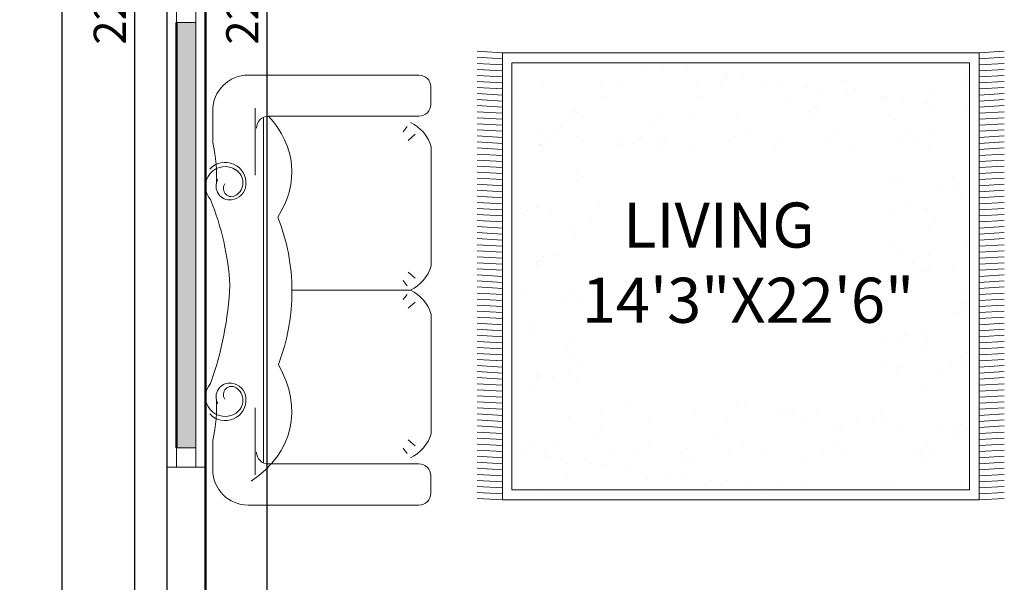
# Model space of a CAD drawing. Units: inches. Extents: x 3064 to 19385, y 846 to 15425.
# Tile 82 of 108: x 7077 to 7230, y 1024 to 1112. Entities that reach past the tile are written whole.
import ezdxf

# ---------------------------------------------------------------- set-up
doc = ezdxf.new("R2010")
doc.units = ezdxf.units.IN
for name, color, linetype, lineweight in [('A-ANNO-DIMS', 2, 'Continuous', 18), ('A-AREA-IDEN', 3, 'Continuous', 18), ('A-FURN', 8, 'Continuous', 18), ('A-GLAZ', 4, 'Continuous', 18), ('A-WALL', 7, 'Continuous', 50), ('C-PROP', 6, 'Continuous', 25)]:
    doc.layers.add(name, color=color, linetype=linetype, lineweight=lineweight)
doc.styles.get("Standard").update_dxf_attribs({"font": 'arial.ttf'})
doc.dimstyles.new('ISO-25', dxfattribs={"dimtxt": 9, "dimasz": 2.5, "dimexe": 1.25, "dimexo": 0.625, "dimtad": 1, "dimdec": 1, "dimlunit": 3, "dimtxsty": 'Standard', "dimcen": 2.5, "dimadec": 0, "dimazin": 0, "dimtfac": 1, "dimtdec": 1, "dimtmove": 0, "dimatfit": 3, "dimfxl": 1, "dimarcsym": 0})

# ---------------------------------------------------------------- blocks, each defined once
blk = doc.blocks.new('*D299')
at = {"layer": 'A-ANNO-DIMS', "color": 0, "lineweight": -2, "transparency": 16777216}
for p, q in [((7099.08, 1252.34), (7093.43, 1252.34)), ((7094.68, 1249.84), (7094.68, 984.84)), ((7105.08, 982.34), (7093.43, 982.34))]:
    blk.add_line(p, q, dxfattribs=at)
at = {"layer": 'A-ANNO-DIMS', "color": 0, "transparency": 16777216}
for points in [[(7094.26, 1249.84), (7095.09, 1249.84), (7094.68, 1252.34)], [(7094.26, 984.84), (7095.09, 984.84), (7094.68, 982.34)]]:
    blk.add_solid(points, dxfattribs=at)
at = {"layer": 'Defpoints', "color": 0, "transparency": 16777216}
for p in [(7099.71, 1252.34), (7094.68, 982.34), (7105.71, 982.34)]:
    blk.add_point(p, dxfattribs=at)
at = {"layer": 'A-ANNO-DIMS', "color": 0, "transparency": 16777216, "insert": (7091.5, 1117.34), "char_height": 5, "attachment_point": 5, "rotation": 90}
blk.add_mtext('22\'-6"', dxfattribs=at)
blk = doc.blocks.new('*D303')
at = {"layer": 'A-ANNO-DIMS', "color": 0, "lineweight": -2, "transparency": 16777216}
for p, q in [((7099.08, 1396.34), (7082.19, 1396.34)), ((7083.44, 882.84), (7083.44, 1393.84)), ((7099.08, 880.34), (7082.19, 880.34))]:
    blk.add_line(p, q, dxfattribs=at)
at = {"layer": 'A-ANNO-DIMS', "color": 0, "transparency": 16777216}
for points in [[(7083.02, 1393.84), (7083.86, 1393.84), (7083.44, 1396.34)], [(7083.02, 882.84), (7083.86, 882.84), (7083.44, 880.34)]]:
    blk.add_solid(points, dxfattribs=at)
at = {"layer": 'Defpoints', "color": 0, "transparency": 16777216}
for p in [(7083.44, 1396.34), (7099.71, 1396.34), (7099.71, 880.34)]:
    blk.add_point(p, dxfattribs=at)
at = {"layer": 'A-ANNO-DIMS', "color": 0, "transparency": 16777216, "insert": (7080.26, 1138.34), "char_height": 5, "attachment_point": 5, "rotation": 90}
blk.add_mtext("43'", dxfattribs=at)
blk = doc.blocks.new('*D223')
at = {"layer": 'A-ANNO-DIMS', "color": 0, "lineweight": -2, "transparency": 16777216}
for p, q in [((7106.33, 1252.34), (7116.51, 1252.34)), ((7115.26, 1249.84), (7115.26, 984.84)), ((7106.33, 982.34), (7116.51, 982.34))]:
    blk.add_line(p, q, dxfattribs=at)
at = {"layer": 'A-ANNO-DIMS', "color": 0, "transparency": 16777216}
for points in [[(7114.84, 1249.84), (7115.67, 1249.84), (7115.26, 1252.34)], [(7114.84, 984.84), (7115.67, 984.84), (7115.26, 982.34)]]:
    blk.add_solid(points, dxfattribs=at)
at = {"layer": 'Defpoints', "color": 0, "transparency": 16777216}
for p in [(7105.71, 1252.34), (7105.71, 982.34), (7115.26, 982.34)]:
    blk.add_point(p, dxfattribs=at)
at = {"layer": 'A-ANNO-DIMS', "color": 0, "transparency": 16777216, "insert": (7112.08, 1117.34), "char_height": 5, "attachment_point": 5, "rotation": 90}
blk.add_mtext('22\'-6"', dxfattribs=at)
blk = doc.blocks.new('carpet-9')
at = {"color": 0, "linetype": 'ByBlock'}
for p, q in [((-2.5225, -0.1423), (-2.5308, 0)), ((-2.4883, -0.1423), (-2.4966, 0)), ((-2.4541, -0.1423), (-2.4624, 0)), ((-2.4199, -0.1423), (-2.4282, 0)), ((-2.3857, -0.1423), (-2.394, 0)), ((-2.3515, -0.1423), (-2.3598, 0)), ((-2.3173, -0.1423), (-2.3256, 0)), ((-2.2831, -0.1423), (-2.2914, 0)), ((-2.2489, -0.1423), (-2.2572, 0)), ((-2.2147, -0.1423), (-2.223, 0)), ((-2.1805, -0.1423), (-2.1888, 0)), ((-2.1463, -0.1423), (-2.1546, 0)), ((-2.1121, -0.1423), (-2.1204, 0)), ((-2.0779, -0.1423), (-2.0862, 0)), ((-2.0437, -0.1423), (-2.052, 0)), ((-2.0095, -0.1423), (-2.0178, 0)), ((-1.9753, -0.1423), (-1.9836, 0)), ((-1.9411, -0.1423), (-1.9494, 0)), ((-1.9069, -0.1423), (-1.9152, 0)), ((-1.8727, -0.1423), (-1.881, 0)), ((-1.8385, -0.1423), (-1.8468, 0)), ((-1.8043, -0.1423), (-1.8126, 0)), ((-1.7701, -0.1423), (-1.7784, 0)), ((-1.7359, -0.1423), (-1.7442, 0)), ((-1.7017, -0.1423), (-1.71, 0)), ((-1.6675, -0.1423), (-1.6758, 0)), ((-1.6333, -0.1423), (-1.6416, 0)), ((-1.5991, -0.1423), (-1.6074, 0)), ((-1.5649, -0.1423), (-1.5732, 0)), ((-1.5307, -0.1423), (-1.539, 0)), ((-1.4965, -0.1423), (-1.5048, 0)), ((-1.4623, -0.1423), (-1.4706, 0)), ((-1.4281, -0.1423), (-1.4364, 0)), ((-1.3939, -0.1423), (-1.4022, 0)), ((-1.3597, -0.1423), (-1.368, 0)), ((-1.3255, -0.1423), (-1.3338, 0)), ((-1.2913, -0.1423), (-1.2996, 0)), ((-1.2571, -0.1423), (-1.2654, 0)), ((-1.2229, -0.1423), (-1.2312, 0)), ((-1.1887, -0.1423), (-1.197, 0)), ((-1.1545, -0.1423), (-1.1628, 0)), ((-1.1203, -0.1423), (-1.1286, 0)), ((-1.0861, -0.1423), (-1.0944, 0)), ((-1.0519, -0.1423), (-1.0602, 0)), ((-1.0177, -0.1423), (-1.026, 0)), ((-0.9835, -0.1423), (-0.9918, 0)), ((-0.9493, -0.1423), (-0.9576, 0)), ((-0.9151, -0.1423), (-0.9234, 0)), ((-0.8809, -0.1423), (-0.8892, 0)), ((-0.8467, -0.1423), (-0.855, 0)), ((-0.8125, -0.1423), (-0.8208, 0)), ((-0.7783, -0.1423), (-0.7866, 0)), ((-0.7441, -0.1423), (-0.7524, 0)), ((-0.7099, -0.1423), (-0.7182, 0)), ((-0.6757, -0.1423), (-0.684, 0)), ((-0.6415, -0.1423), (-0.6498, 0)), ((-0.6073, -0.1423), (-0.6156, 0)), ((-0.5731, -0.1423), (-0.5814, 0)), ((-0.5389, -0.1423), (-0.5472, 0)), ((-0.5047, -0.1423), (-0.513, 0)), ((-0.4705, -0.1423), (-0.4788, 0)), ((-0.4363, -0.1423), (-0.4446, 0)), ((-0.4021, -0.1423), (-0.4104, 0)), ((-0.3679, -0.1423), (-0.3762, 0)), ((-0.3337, -0.1423), (-0.342, 0)), ((-0.2995, -0.1423), (-0.3078, 0)), ((-0.2653, -0.1423), (-0.2736, 0)), ((-0.2311, -0.1423), (-0.2394, 0)), ((-0.1969, -0.1423), (-0.2052, 0)), ((-0.1627, -0.1423), (-0.171, 0)), ((-0.1285, -0.1423), (-0.1368, 0)), ((-0.0943, -0.1423), (-0.1026, 0)), ((-0.0601, -0.1423), (-0.0684, 0)), ((-0.0259, -0.1423), (-0.0342, 0)), ((0.0083, -0.1423), (0, 0)), ((0.0081, -0.1423), (-2.5225, -0.1423)), ((-2.5225, -0.1423), (-2.5225, -2.8423)), ((0.0081, -2.8423), (0.0081, -0.1423)), ((-0.0489, -0.1963), (-2.4655, -0.1963)), ((-2.4655, -0.1963), (-2.4655, -2.7883)), ((-2.3955, -0.2124), (-2.3955, -0.2124)), ((-2.2062, -0.2078), (-2.2062, -0.2078)), ((-1.4511, -0.2068), (-1.4511, -0.2068)), ((-1.1079, -0.2175), (-1.1079, -0.2175)), ((-0.8244, -0.2203), (-0.8244, -0.2203)), ((-0.0489, -2.7883), (-0.0489, -0.1963)), ((-2.3654, -0.2435), (-2.3654, -0.2435)), ((-1.7544, -0.2756), (-1.7544, -0.2756)), ((-1.7121, -0.2501), (-1.7121, -0.2501)), ((-1.1533, -0.2312), (-1.1533, -0.2312)), ((-1.0792, -0.2355), (-1.0792, -0.2355)), ((-1.0491, -0.2666), (-1.0491, -0.2666)), ((-0.7647, -0.2281), (-0.7647, -0.2281)), ((-0.4215, -0.2387), (-0.4215, -0.2387)), ((-0.3958, -0.2731), (-0.3958, -0.2731)), ((-0.0783, -0.2494), (-0.0783, -0.2494)), ((-1.8205, -0.2931), (-1.8205, -0.2931)), ((-1.2958, -0.294), (-1.2958, -0.294)), ((-0.7551, -0.2963), (-0.7551, -0.2963)), ((-0.3726, -0.2881), (-0.3726, -0.2881)), ((-1.7666, -0.3634), (-1.7666, -0.3634)), ((-0.7072, -0.3675), (-0.7072, -0.3675)), ((-0.3848, -0.3759), (-0.3848, -0.3759)), ((-2.3219, -0.4132), (-2.3219, -0.4132)), ((-2.2381, -0.437), (-2.2381, -0.437)), ((-2.203, -0.4115), (-2.203, -0.4115)), ((-2.0942, -0.413), (-2.0942, -0.413)), ((-1.9787, -0.4238), (-1.9787, -0.4238)), ((-1.6355, -0.4344), (-1.6355, -0.4344)), ((-1.5701, -0.3969), (-1.5701, -0.3969)), ((-1.54, -0.428), (-1.54, -0.428)), ((-1.3744, -0.4294), (-1.3744, -0.4294)), ((-1.3149, -0.4312), (-1.3149, -0.4312)), ((-1.2923, -0.4451), (-1.2923, -0.4451)), ((-0.8867, -0.4345), (-0.8867, -0.4345)), ((-0.3091, -0.4326), (-0.3091, -0.4326)), ((-0.2538, -0.4199), (-0.2538, -0.4199)), ((-2.0464, -0.4841), (-2.0464, -0.4841)), ((-0.949, -0.4557), (-0.949, -0.4557)), ((-0.8562, -0.4496), (-0.8562, -0.4496)), ((-0.6058, -0.4663), (-0.6058, -0.4663)), ((-0.2626, -0.477), (-0.2626, -0.477)), ((-0.2237, -0.451), (-0.2237, -0.451)), ((-1.6482, -0.5493), (-1.6482, -0.5493)), ((-1.3271, -0.519), (-1.3271, -0.519)), ((-0.2612, -0.5038), (-0.2612, -0.5038)), ((-2.2571, -0.5742), (-2.2571, -0.5742)), ((-2.061, -0.5583), (-2.061, -0.5583)), ((-2.0309, -0.5894), (-2.0309, -0.5894)), ((-1.7985, -0.5926), (-1.7985, -0.5926)), ((-1.3776, -0.5959), (-1.3776, -0.5959)), ((-0.9284, -0.5657), (-0.9284, -0.5657)), ((-0.8753, -0.5867), (-0.8753, -0.5867)), ((-0.7447, -0.5813), (-0.7447, -0.5813)), ((-0.7146, -0.6124), (-0.7146, -0.6124)), ((-0.4167, -0.6051), (-0.4167, -0.6051)), ((-2.2693, -0.6621), (-2.2693, -0.6621)), ((-2.1435, -0.6273), (-2.1435, -0.6273)), ((-1.8003, -0.6379), (-1.8003, -0.6379)), ((-1.6003, -0.6204), (-1.6003, -0.6204)), ((-1.4571, -0.6486), (-1.4571, -0.6486)), ((-1.1139, -0.6592), (-1.1139, -0.6592)), ((-0.0613, -0.619), (-0.0613, -0.619)), ((-2.2675, -0.6823), (-2.2675, -0.6823)), ((-1.2021, -0.6856), (-1.2021, -0.6856)), ((-0.8875, -0.6746), (-0.8875, -0.6746)), ((-0.7706, -0.6698), (-0.7706, -0.6698)), ((-0.4823, -0.702), (-0.4823, -0.702)), ((-0.4274, -0.6805), (-0.4274, -0.6805)), ((-0.0842, -0.6911), (-0.0842, -0.6911)), ((-0.4357, -0.7423), (-0.4357, -0.7423)), ((-0.4479, -0.8302), (-0.4479, -0.8302)), ((-2.3197, -0.8449), (-2.3197, -0.8449)), ((-2.3012, -0.8913), (-2.3012, -0.8913)), ((-1.9765, -0.8555), (-1.9765, -0.8555)), ((-2.3593, -0.9188), (-2.3593, -0.9188)), ((-2.0952, -0.9385), (-2.0952, -0.9385)), ((-0.4101, -0.9272), (-0.4101, -0.9272)), ((-0.2604, -0.9086), (-0.2604, -0.9086)), ((-0.3801, -0.9583), (-0.3801, -0.9583)), ((-0.3101, -0.9581), (-0.3101, -0.9581)), ((-2.3203, -1.0285), (-2.3203, -1.0285)), ((-2.0474, -1.0097), (-2.0474, -1.0097)), ((-0.2622, -1.0293), (-0.2622, -1.0293)), ((-2.2173, -1.0656), (-2.2173, -1.0656)), ((-2.1872, -1.0967), (-2.1872, -1.0967)), ((-2.1608, -1.0831), (-2.1608, -1.0831)), ((-0.4798, -1.0594), (-0.4798, -1.0594)), ((-2.3325, -1.1163), (-2.3325, -1.1163)), ((-0.4448, -1.1362), (-0.4448, -1.1362)), ((-0.2176, -1.1263), (-0.2176, -1.1263)), ((-0.1015, -1.1469), (-0.1015, -1.1469)), ((-2.2685, -1.2078), (-2.2685, -1.2078)), ((-0.4989, -1.1966), (-0.4989, -1.1966)), ((-2.0248, -1.2646), (-2.0248, -1.2646)), ((-0.4833, -1.2275), (-0.4833, -1.2275)), ((-0.0756, -1.2731), (-0.0756, -1.2731)), ((-2.3257, -1.2866), (-2.3257, -1.2866)), ((-1.9824, -1.2972), (-1.9824, -1.2972)), ((-0.5111, -1.2844), (-0.5111, -1.2844)), ((-2.3643, -1.3455), (-2.3643, -1.3455)), ((-0.2664, -1.3504), (-0.2664, -1.3504)), ((-0.0593, -1.3522), (-0.0593, -1.3522)), ((-0.0715, -1.44), (-0.0715, -1.44)), ((-2.3834, -1.4827), (-2.3834, -1.4827)), ((-2.0963, -1.464), (-2.0963, -1.464)), ((-0.5364, -1.4656), (-0.5364, -1.4656)), ((-0.3111, -1.4836), (-0.3111, -1.4836)), ((-2.1587, -1.5148), (-2.1587, -1.5148)), ((-2.0484, -1.5352), (-2.0484, -1.5352)), ((-0.5429, -1.5136), (-0.5429, -1.5136)), ((-0.2632, -1.5548), (-0.2632, -1.5548)), ((-2.3956, -1.5705), (-2.3956, -1.5705)), ((-2.3737, -1.5729), (-2.3737, -1.5729)), ((-2.3436, -1.604), (-2.3436, -1.604)), ((-0.4426, -1.5679), (-0.4426, -1.5679)), ((-0.0994, -1.5785), (-0.0994, -1.5785)), ((-0.3739, -1.6336), (-0.3739, -1.6336)), ((-0.1033, -1.6692), (-0.1033, -1.6692)), ((-2.343, -1.7423), (-2.343, -1.7423)), ((-2.2695, -1.7333), (-2.2695, -1.7333)), ((-2.1811, -1.7719), (-2.1811, -1.7719)), ((-1.9998, -1.753), (-1.9998, -1.753)), ((-0.4843, -1.753), (-0.4843, -1.753)), ((-0.2319, -1.7804), (-0.2319, -1.7804)), ((-2.4274, -1.7997), (-2.4274, -1.7997)), ((-0.2837, -1.8061), (-0.2837, -1.8061)), ((-0.2018, -1.8115), (-0.2018, -1.8115)), ((-0.1224, -1.8064), (-0.1224, -1.8064)), ((-0.1346, -1.8942), (-0.1346, -1.8942)), ((-2.4465, -1.9369), (-2.4465, -1.9369)), ((-2.0391, -1.9187), (-2.0391, -1.9187)), ((-2.009, -1.9498), (-2.009, -1.9498)), ((-2.1646, -1.9565), (-2.1646, -1.9565)), ((-2.0973, -1.9895), (-2.0973, -1.9895)), ((-1.9879, -1.9553), (-1.9879, -1.9553)), ((-2.4587, -2.0248), (-2.4587, -2.0248)), ((-2.0494, -2.0607), (-2.0494, -2.0607)), ((-0.4485, -2.0096), (-0.4485, -2.0096)), ((-0.3121, -2.0092), (-0.3121, -2.0092)), ((-0.1053, -2.0203), (-0.1053, -2.0203)), ((-2.0069, -2.0925), (-2.0069, -2.0925)), ((-0.2642, -2.0803), (-0.2642, -2.0803)), ((-2.3408, -2.174), (-2.3408, -2.174)), ((-0.5303, -2.1409), (-0.5303, -2.1409)), ((-0.1665, -2.1234), (-0.1665, -2.1234)), ((-2.0191, -2.1804), (-2.0191, -2.1804)), ((-1.9976, -2.1847), (-1.9976, -2.1847)), ((-2.3374, -2.2792), (-2.3374, -2.2792)), ((-2.2705, -2.2589), (-2.2705, -2.2589)), ((-0.4854, -2.2785), (-0.4854, -2.2785)), ((-0.2815, -2.2378), (-0.2815, -2.2378)), ((-0.1855, -2.2606), (-0.1855, -2.2606)), ((-1.6745, -2.2957), (-1.6745, -2.2957)), ((-1.5796, -2.3359), (-1.5796, -2.3359)), ((-1.1573, -2.3333), (-1.1573, -2.3333)), ((-1.0211, -2.3023), (-1.0211, -2.3023)), ((-0.3883, -2.2877), (-0.3883, -2.2877)), ((-0.3582, -2.3188), (-0.3582, -2.3188)), ((-1.8245, -2.3951), (-1.8245, -2.3951)), ((-0.1977, -2.3485), (-0.1977, -2.3485)), ((-2.1954, -2.426), (-2.1954, -2.426)), ((-2.1819, -2.4122), (-2.1819, -2.4122)), ((-2.051, -2.4096), (-2.051, -2.4096)), ((-1.8387, -2.4229), (-1.8387, -2.4229)), ((-1.4955, -2.4335), (-1.4955, -2.4335)), ((-1.1523, -2.4441), (-1.1523, -2.4441)), ((-1.1278, -2.4037), (-1.1278, -2.4037)), ((-0.8791, -2.4491), (-0.8791, -2.4491)), ((-0.7591, -2.3984), (-0.7591, -2.3984)), ((-0.6692, -2.4221), (-0.6692, -2.4221)), ((-2.1654, -2.4571), (-2.1654, -2.4571)), ((-1.512, -2.4637), (-1.512, -2.4637)), ((-1.14, -2.4915), (-1.14, -2.4915)), ((-0.8491, -2.4802), (-0.8491, -2.4802)), ((-0.8091, -2.4548), (-0.8091, -2.4548)), ((-0.7113, -2.4695), (-0.7113, -2.4695)), ((-0.4659, -2.4654), (-0.4659, -2.4654)), ((-0.1957, -2.4867), (-0.1957, -2.4867)), ((-0.1226, -2.476), (-0.1226, -2.476)), ((-2.0983, -2.515), (-2.0983, -2.515)), ((-2.0701, -2.5468), (-2.0701, -2.5468)), ((-1.3785, -2.5314), (-1.3785, -2.5314)), ((-0.6882, -2.5593), (-0.6882, -2.5593)), ((-0.3131, -2.5347), (-0.3131, -2.5347)), ((-2.3468, -2.6157), (-2.3468, -2.6157)), ((-2.0504, -2.5862), (-2.0504, -2.5862)), ((-1.6114, -2.5652), (-1.6114, -2.5652)), ((-1.37, -2.6105), (-1.37, -2.6105)), ((-0.2652, -2.6058), (-0.2652, -2.6058)), ((-0.2296, -2.5777), (-0.2296, -2.5777)), ((-2.0823, -2.6346), (-2.0823, -2.6346)), ((-2.0035, -2.6264), (-2.0035, -2.6264)), ((-2.0029, -2.6251), (-2.0029, -2.6251)), ((-1.6603, -2.637), (-1.6603, -2.637)), ((-1.6522, -2.6513), (-1.6522, -2.6513)), ((-1.3399, -2.6416), (-1.3399, -2.6416)), ((-1.3171, -2.6476), (-1.3171, -2.6476)), ((-0.9739, -2.6583), (-0.9739, -2.6583)), ((-0.9324, -2.6677), (-0.9324, -2.6677)), ((-0.7004, -2.6471), (-0.7004, -2.6471)), ((-0.6866, -2.6481), (-0.6866, -2.6481)), ((-0.6307, -2.6689), (-0.6307, -2.6689)), ((-0.0537, -2.6335), (-0.0537, -2.6335)), ((-1.6305, -2.7023), (-1.6305, -2.7023)), ((-1.6044, -2.7225), (-1.6044, -2.7225)), ((-1.1719, -2.7207), (-1.1719, -2.7207)), ((-0.2875, -2.6795), (-0.2875, -2.6795)), ((-0.2487, -2.7149), (-0.2487, -2.7149)), ((-2.2715, -2.7844), (-2.2715, -2.7844)), ((-1.8609, -2.7719), (-1.8609, -2.7719)), ((-1.2062, -2.7876), (-1.2062, -2.7876)), ((-2.5225, -2.8423), (-2.5308, -2.9845)), ((-2.5225, -2.8423), (0.0081, -2.8423)), ((-2.4883, -2.8423), (-2.4966, -2.9845)), ((-2.4655, -2.7883), (-0.0489, -2.7883)), ((-2.4541, -2.8423), (-2.4624, -2.9845)), ((-2.4199, -2.8423), (-2.4282, -2.9845)), ((-2.3857, -2.8423), (-2.394, -2.9845)), ((-2.3515, -2.8423), (-2.3598, -2.9845)), ((-2.3173, -2.8423), (-2.3256, -2.9845)), ((-2.2831, -2.8423), (-2.2914, -2.9845)), ((-2.2489, -2.8423), (-2.2572, -2.9845)), ((-2.2147, -2.8423), (-2.223, -2.9845)), ((-2.1805, -2.8423), (-2.1888, -2.9845)), ((-2.1463, -2.8423), (-2.1546, -2.9845)), ((-2.1121, -2.8423), (-2.1204, -2.9845)), ((-2.0779, -2.8423), (-2.0862, -2.9845)), ((-2.0437, -2.8423), (-2.052, -2.9845)), ((-2.0095, -2.8423), (-2.0178, -2.9845)), ((-1.9753, -2.8423), (-1.9836, -2.9845)), ((-1.9411, -2.8423), (-1.9494, -2.9845)), ((-1.9069, -2.8423), (-1.9152, -2.9845)), ((-1.8727, -2.8423), (-1.881, -2.9845)), ((-1.8385, -2.8423), (-1.8468, -2.9845)), ((-1.8043, -2.8423), (-1.8126, -2.9845)), ((-1.7701, -2.8423), (-1.7784, -2.9845)), ((-1.7359, -2.8423), (-1.7442, -2.9845)), ((-1.7017, -2.8423), (-1.71, -2.9845)), ((-1.6675, -2.8423), (-1.6758, -2.9845)), ((-1.6333, -2.8423), (-1.6416, -2.9845)), ((-1.5991, -2.8423), (-1.6074, -2.9845)), ((-1.5649, -2.8423), (-1.5732, -2.9845)), ((-1.5307, -2.8423), (-1.539, -2.9845)), ((-1.4965, -2.8423), (-1.5048, -2.9845)), ((-1.4623, -2.8423), (-1.4706, -2.9845)), ((-1.4281, -2.8423), (-1.4364, -2.9845)), ((-1.3939, -2.8423), (-1.4022, -2.9845)), ((-1.3597, -2.8423), (-1.368, -2.9845)), ((-1.3255, -2.8423), (-1.3338, -2.9845)), ((-1.2913, -2.8423), (-1.2996, -2.9845)), ((-1.2571, -2.8423), (-1.2654, -2.9845)), ((-1.2229, -2.8423), (-1.2312, -2.9845)), ((-1.1887, -2.8423), (-1.197, -2.9845)), ((-1.1545, -2.8423), (-1.1628, -2.9845)), ((-1.1203, -2.8423), (-1.1286, -2.9845)), ((-1.0861, -2.8423), (-1.0944, -2.9845)), ((-1.0519, -2.8423), (-1.0602, -2.9845)), ((-1.0177, -2.8423), (-1.026, -2.9845)), ((-0.9835, -2.8423), (-0.9918, -2.9845)), ((-0.9493, -2.8423), (-0.9576, -2.9845)), ((-0.9151, -2.8423), (-0.9234, -2.9845)), ((-0.8809, -2.8423), (-0.8892, -2.9845)), ((-0.8467, -2.8423), (-0.855, -2.9845)), ((-0.8125, -2.8423), (-0.8208, -2.9845)), ((-0.7783, -2.8423), (-0.7866, -2.9845)), ((-0.7441, -2.8423), (-0.7524, -2.9845)), ((-0.7099, -2.8423), (-0.7182, -2.9845)), ((-0.6757, -2.8423), (-0.684, -2.9845)), ((-0.6415, -2.8423), (-0.6498, -2.9845)), ((-0.6073, -2.8423), (-0.6156, -2.9845)), ((-0.5731, -2.8423), (-0.5814, -2.9845)), ((-0.5389, -2.8423), (-0.5472, -2.9845)), ((-0.5047, -2.8423), (-0.513, -2.9845)), ((-0.4705, -2.8423), (-0.4788, -2.9845)), ((-0.4363, -2.8423), (-0.4446, -2.9845)), ((-0.4021, -2.8423), (-0.4104, -2.9845)), ((-0.3679, -2.8423), (-0.3762, -2.9845)), ((-0.3337, -2.8423), (-0.342, -2.9845)), ((-0.2995, -2.8423), (-0.3078, -2.9845)), ((-0.2653, -2.8423), (-0.2736, -2.9845)), ((-0.2311, -2.8423), (-0.2394, -2.9845)), ((-0.1969, -2.8423), (-0.2052, -2.9845)), ((-0.1627, -2.8423), (-0.171, -2.9845)), ((-0.1285, -2.8423), (-0.1368, -2.9845)), ((-0.0943, -2.8423), (-0.1026, -2.9845)), ((-0.0601, -2.8423), (-0.0684, -2.9845)), ((-0.0259, -2.8423), (-0.0342, -2.9845)), ((0.0083, -2.8423), (0, -2.9845))]:
    blk.add_line(p, q, dxfattribs=at)
blk = doc.blocks.new('sofa-33')
at = {"color": 0, "linetype": 'ByBlock'}
for p, q in [((-0.026, 0.9238), (-0.1, 0.9238)), ((0.657, 0.9252), (0.1531, 0.9252)), ((0.8633, 0.9252), (1.3671, 0.9252)), ((1.6203, 0.9238), (1.5463, 0.9238)), ((-0.15, 0.15), (-0.15, 0.8738)), ((0.024, 0.2361), (0.024, 0.8738)), ((0.05, 0.8375), (0.05, 0.8379)), ((0.1006, 0.8574), (0.1265, 0.8286)), ((0.7096, 0.8574), (0.6837, 0.8286)), ((0.7602, 0.8375), (0.7601, 0.8379)), ((0.7601, 0.8375), (0.7601, 0.8379)), ((0.7602, 0.8375), (0.7602, 0.3356)), ((0.8107, 0.8574), (0.8366, 0.8286)), ((1.4197, 0.8574), (1.3938, 0.8286)), ((1.4702, 0.8375), (1.4703, 0.8379)), ((1.4702, 0.8375), (1.4703, 0.8379)), ((1.4963, 0.2361), (1.4963, 0.8738)), ((1.6703, 0.15), (1.6703, 0.8738)), ((0.0903, 0.8062), (0.0682, 0.8242)), ((0.7199, 0.8062), (0.742, 0.8242)), ((0.8004, 0.8062), (0.7783, 0.8242)), ((1.43, 0.8062), (1.4521, 0.8242)), ((0.0289, 0.2145), (1.4914, 0.2145)), ((-0.01, 0.1801), (0.2738, 0.1801)), ((1.5422, 0.1801), (1.2585, 0.1801)), ((0, 0), (0.1356, 0)), ((1.5322, 0), (1.3966, 0))]:
    blk.add_line(p, q, dxfattribs=at)
at = {"color": 0, "linetype": 'ByBlock', "extrusion": (0, 0, -1)}
for centre, major_axis, ratio, start_param, end_param in [((-0.1, 0.8738), (0.0354, 0.0354), 1, 3.926992, 5.497787), ((-0.026, 0.8738), (-0.0354, 0.0354), 1, 0.785398, 2.356196), ((0.1997, 0.7661), (0.1173, 0.1173), 1, 4.372209, 5.213218), ((0.6105, 0.7661), (0.1173, 0.1173), 1, -0.500829, 0.34018), ((0.9098, 0.7661), (0.1173, 0.1173), 1, 4.372209, 5.213218), ((1.3206, 0.7661), (-0.1173, 0.1173), 1, 1.069968, 1.910976), ((1.5463, 0.8738), (-0.0354, 0.0354), 1, 5.497786, 7.068583), ((1.6203, 0.8738), (0.0354, 0.0354), 1, -0.785398, 0.785398), ((1.147, -0.5336), (0.1998, 0.8608), 0.59532, -0.502747, 0.502747), ((0.3234, -0.6657), (-0.0931, 0.9998), 0.551284, -0.397889, 0.397889), ((0.7664, -0.6685), (-0.0034, 1.0041), 0.922365, -0.343589, 0.343589), ((0.074, 0.2361), (-0.0354, 0.0354), 1, 3.926991, 5.497788), ((1.4463, 0.2361), (0.0354, 0.0354), 1, 0.785397, 2.356194), ((0, 0.15), (0.1061, 0.1061), 1, 2.356194, 3.926992), ((0.3076, 0.0525), (-0.0624, 0.0624), 1, 4.675944, 7.152385), ((0.3052, 0.0629), (-0.0458, 0.0458), 1, 6.094039, 8.043134), ((0.3092, 0.0712), (0.0491, 0.0491), 1, -0.701597, 0.659711), ((1.223, 0.0712), (-0.0491, 0.0491), 1, 5.623477, 6.984784), ((1.227, 0.0629), (0.0458, 0.0458), 1, 4.52324, 6.472335), ((1.2246, 0.0525), (-0.0624, 0.0624), 1, 0.701599, 3.17804), ((1.5203, 0.15), (0.1061, 0.1061), 1, 0.785398, 2.356194), ((0.3208, 0.0524), (-0.059, 0.059), 1, 3.186406, 6.094039), ((0.3301, 0.0798), (0.0245, 0.0245), 1, 0.189152, 2.952444), ((1.2115, 0.0524), (0.059, 0.059), 1, 0.189149, 3.096782), ((1.2022, 0.0798), (0.0245, 0.0245), 1, 1.759947, 4.52324), ((0.3201, 0.0726), (-0.0414, 0.0414), 1, 2.230507, 4.423483), ((0.8779, -1.3822), (-0.3228, 1.4289), 0.878591, -0.144977, 0.144977), ((0.6669, -1.3904), (1.0359, 1.0359), 1, 5.547613, 5.837566), ((1.2122, 0.0726), (-0.0414, 0.0414), 1, 3.430501, 5.623477), ((0.2824, -0.6613), (-0.479, 0.479), 1, 0.566947, 0.842011), ((1.2498, -0.6613), (0.479, 0.479), 1, 5.441177, 5.716241)]:
    blk.add_ellipse(centre, major_axis=major_axis, ratio=ratio, start_param=start_param, end_param=end_param, dxfattribs=at)
blk = doc.blocks.new('WIN-1900')
blk.add_line((3, 0), (3, 66))
blk.add_lwpolyline([(3, 66), (0, 66), (0, 69), (3, 69)], close=True)

msp = doc.modelspace()

# ---------------------------------------------------------------- hatches: boundary and pattern name
at = {"layer": 'A-GLAZ'}
h = msp.add_hatch(color=256, dxfattribs=at)
h.dxf.hatch_style = 1
h.paths.add_polyline_path([(7101.21, 1045.34), (7104.21, 1045.34), (7104.21, 1111.34), (7101.21, 1111.34)])

# ---------------------------------------------------------------- linework, layer by layer
msp.add_line((7105.71, 1042.34), (7099.71, 1042.34), dxfattribs=at)
msp.add_lwpolyline([(7104.21, 1042.34), (7101.21, 1042.34), (7101.21, 1045.34), (7104.21, 1045.34)], close=True, dxfattribs=at)
at = {"layer": 'A-WALL'}
for p, q in [((7105.71, 1390.34), (7105.71, 982.34)), ((7101.21, 1045.34), (7101.21, 1111.34))]:
    msp.add_line(p, q, dxfattribs=at)
at = {"layer": 'C-PROP'}
msp.add_line((7099.71, 1396.34), (7099.71, 880.34), dxfattribs=at)

# ---------------------------------------------------------------- block references
at = {"layer": 'A-FURN', "rotation": 270}
for name, p, xscale, yscale, zscale in [('carpet-9', (7229.79, 1037.48), 27.43020644299853, 27.43020644299853, 27.43020644299853), ('sofa-33', (7106.84, 1097.7), 36.66436083614781, 36.66436083614781, 36.66436083614781)]:
    msp.add_blockref(name, p, dxfattribs=dict(at, xscale=xscale, yscale=yscale, zscale=zscale))
at = {"layer": 'A-GLAZ'}
msp.add_blockref('WIN-1900', (7101.2, 1045.34), dxfattribs=at)

# ---------------------------------------------------------------- texts
at = {"layer": 'A-AREA-IDEN', "insert": (7164.16, 1083.42), "char_height": 7, "attachment_point": 1}
msp.add_mtext_dynamic_manual_height_columns('   LIVING\\P14\'3"X22\'6"', width=67.5924, gutter_width=12.5, heights=[0], dxfattribs=at)

# ---------------------------------------------------------------- dimensions: what is measured, and where the dimension line sits
at = {"layer": 'A-ANNO-DIMS'}
for base, p1, p2, override, picture, middle in [((7083.44, 1396.34), (7099.71, 880.34), (7099.71, 1396.34), {"dimtxt": 5, "dimclrd": 0, "dimclre": 0, "dimclrt": 0}, '*D303', (7080.26, 1138.34)), ((7094.68, 982.34), (7099.71, 1252.34), (7105.71, 982.34), {"dimtxt": 5, "dimclrd": 0, "dimclre": 0, "dimclrt": 0, "dimtmove": 1}, '*D299', (7091.5, 1117.34)), ((7115.26, 982.34), (7105.71, 1252.34), (7105.71, 982.34), {"dimtxt": 5, "dimclrd": 0, "dimclre": 0, "dimclrt": 0}, '*D223', (7112.08, 1117.34))]:
    dim = msp.add_linear_dim(base=base, p1=p1, p2=p2, angle=90, dimstyle='ISO-25', override=override, dxfattribs=at)
    dim.commit()
    dim.dimension.update_dxf_attribs({"geometry": picture, "text_midpoint": middle})

doc.saveas('drawing.dxf')
